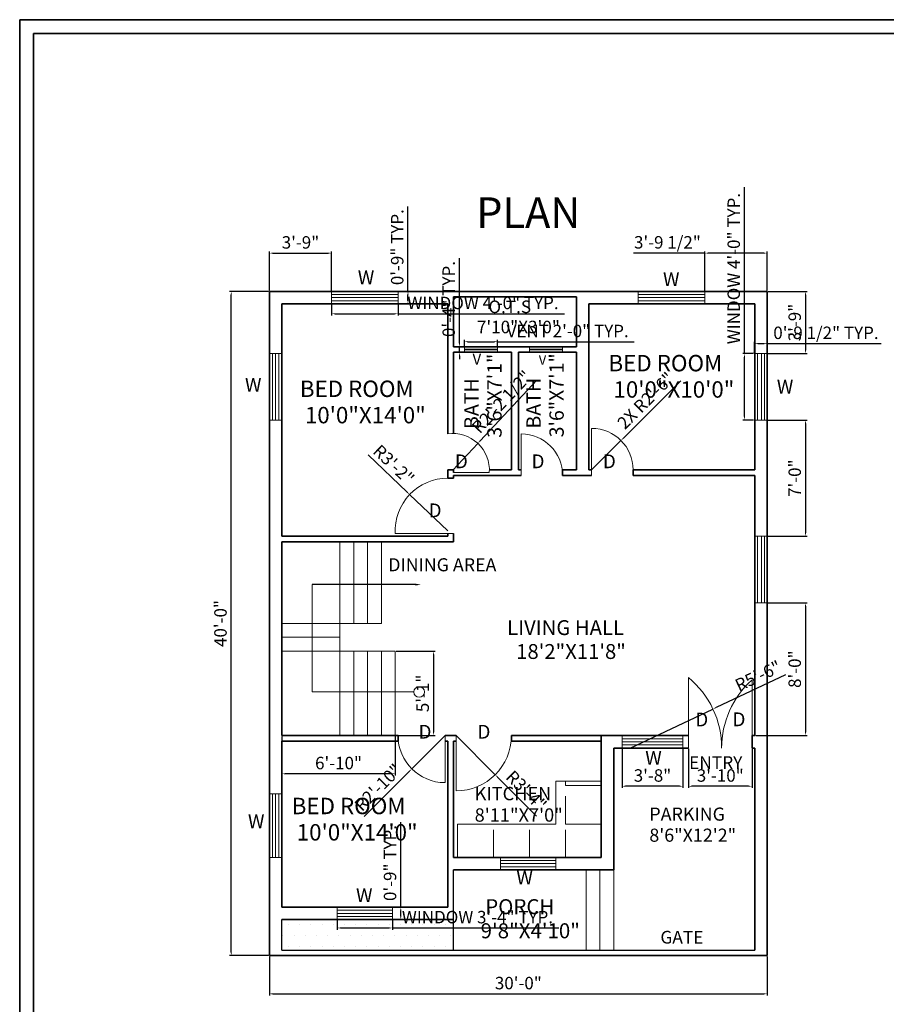
# Model space of a CAD drawing. Units: inches. Extents: x 2413 to 4117, y 1127 to 2321.
# Tile 3 of 5: x 2413 to 3039, y 1610 to 2321. Entities that reach past the tile are written whole.
import ezdxf
from ezdxf import colors
from ezdxf.entities.mleader import LeaderData, LeaderLine
from ezdxf.math import Vec2, Vec3

# ---------------------------------------------------------------- set-up
doc = ezdxf.new("R2010")
doc.units = ezdxf.units.IN
doc.linetypes.add('ACAD_ISO02W100', pattern=[15, 12, -3])
doc.linetypes.add('ACAD_ISO03W100', pattern=[30, 12, -18])
doc.layers.get('Defpoints').update_dxf_attribs({"linetype": 'ACAD_ISO03W100'})
for name, color, linetype, lineweight in [('A-ANNO-DIMS', 2, 'Continuous', 18), ('A-ANNO-SYMB', 2, 'Continuous', 18), ('A-ANNO-TEXT', 7, 'Continuous', 18), ('A-ANNO-TITL', 7, 'Continuous', 30), ('A-ANNO-TTLB', 7, 'Continuous', 35), ('A-AREA-IDEN', 7, 'Continuous', 18), ('A-DOOR', 3, 'Continuous', 20), ('A-FLOR', 7, 'Continuous', 30), ('A-FLOR-FIXT', 8, 'Continuous', 18), ('A-FLOR-OVHD', 8, 'ACAD_ISO02W100', 18), ('A-FLOR-PATT', 4, 'Continuous', 13), ('A-FLOR-STRS', 3, 'Continuous', 20), ('A-GLAZ', 4, 'Continuous', 18), ('A-WALL', 7, 'Continuous', 35)]:
    doc.layers.add(name, color=color, linetype=linetype, lineweight=lineweight)
doc.styles.get("Standard").update_dxf_attribs({"font": 'arial.ttf'})
doc.dimstyles.new('ISO-25', dxfattribs={"dimtxt": 9, "dimasz": 2.5, "dimexe": 1.25, "dimexo": 0.625, "dimgap": 2, "dimtad": 1, "dimdec": 1, "dimlunit": 4, "dimtxsty": 'Standard', "dimcen": 2.5, "dimazin": 0, "dimtfac": 1, "dimtdec": 1, "dimtmove": 0, "dimatfit": 3, "dimfxl": 1, "dimarcsym": 0})

# ---------------------------------------------------------------- blocks, each defined once
blk = doc.blocks.new('WIN-48-PLAN')
for p, q in [((0, 9), (0, 0)), ((48, 9), (48, 0)), ((0, 6.75), (48, 6.75)), ((0, 4.5), (48, 4.5)), ((0, 2.25), (48, 2.25))]:
    blk.add_line(p, q)
blk = doc.blocks.new('WIN-40-PLAN')
for p, q in [((0, 0), (0, 9)), ((40, 0), (40, 9)), ((0, 6.75), (40, 6.75)), ((0, 4.5), (40, 4.5)), ((0, 2.25), (40, 2.25))]:
    blk.add_line(p, q)
blk = doc.blocks.new('VENT-24-PLAN')
for p, q in [((0, 0), (0, 4)), ((0, 2.25), (24, 2.25)), ((0, 1.75), (24, 1.75)), ((24, 0), (24, 4))]:
    blk.add_line(p, q)
blk = doc.blocks.new('WIN-48-SIDE-PLAN')
for p, q in [((0, 48), (9.25, 48)), ((2.25, 48), (2.25, 0)), ((5, 48), (5, 0)), ((7.25, 48), (7.25, 0)), ((0, 0), (9.25, 0))]:
    blk.add_line(p, q)
blk = doc.blocks.new('*D16')
at = {"layer": 'A-ANNO-DIMS', "color": 0, "lineweight": -2, "transparency": 16777216}
for p, q in [((2638.17, 2115.41), (2638.17, 2107.58)), ((2686.17, 2115.41), (2686.17, 2107.58)), ((2640.67, 2108.83), (2683.67, 2108.83)), ((2686.17, 2108.83), (2806.56, 2108.83))]:
    blk.add_line(p, q, dxfattribs=at)
at = {"layer": 'A-ANNO-DIMS', "color": 0, "transparency": 16777216}
for points in [[(2640.67, 2109.25), (2640.67, 2108.42), (2638.17, 2108.83)], [(2683.67, 2109.25), (2683.67, 2108.42), (2686.17, 2108.83)]]:
    blk.add_solid(points, dxfattribs=at)
at = {"layer": 'Defpoints', "color": 0, "transparency": 16777216}
for p in [(2638.17, 2116.03), (2686.17, 2116.03), (2686.17, 2108.83)]:
    blk.add_point(p, dxfattribs=at)
at = {"layer": 'A-ANNO-DIMS', "color": 0, "transparency": 16777216, "insert": (2747.61, 2115.49), "char_height": 9, "attachment_point": 5}
blk.add_mtext('WINDOW 4\'-0" TYP.', dxfattribs=at)
blk = doc.blocks.new('*D17')
at = {"layer": 'A-ANNO-DIMS', "color": 0, "lineweight": -2, "transparency": 16777216}
for p, q in [((2693.37, 2125.03), (2693.37, 2186.39)), ((2686.79, 2125.03), (2694.62, 2125.03)), ((2693.37, 2118.53), (2693.37, 2122.53)), ((2686.79, 2116.03), (2694.62, 2116.03))]:
    blk.add_line(p, q, dxfattribs=at)
at = {"layer": 'A-ANNO-DIMS', "color": 0, "transparency": 16777216}
for points in [[(2692.95, 2122.53), (2693.79, 2122.53), (2693.37, 2125.03)], [(2692.95, 2118.53), (2693.79, 2118.53), (2693.37, 2116.03)]]:
    blk.add_solid(points, dxfattribs=at)
at = {"layer": 'Defpoints', "color": 0, "transparency": 16777216}
for p in [(2686.17, 2125.03), (2693.37, 2125.03), (2686.17, 2116.03)]:
    blk.add_point(p, dxfattribs=at)
at = {"layer": 'A-ANNO-DIMS', "color": 0, "transparency": 16777216, "insert": (2686.77, 2156.96), "char_height": 9, "attachment_point": 5, "rotation": 90}
blk.add_mtext('0\'-9" TYP.', dxfattribs=at)
blk = doc.blocks.new('*D18')
at = {"layer": 'A-ANNO-DIMS', "color": 0, "lineweight": -2, "transparency": 16777216}
for p, q in [((2642.17, 1670.41), (2642.17, 1663.78)), ((2644.67, 1665.03), (2679.67, 1665.03)), ((2682.17, 1670.41), (2682.17, 1663.78)), ((2682.17, 1665.03), (2802.56, 1665.03))]:
    blk.add_line(p, q, dxfattribs=at)
at = {"layer": 'A-ANNO-DIMS', "color": 0, "transparency": 16777216}
for points in [[(2644.67, 1665.45), (2644.67, 1664.62), (2642.17, 1665.03)], [(2679.67, 1665.45), (2679.67, 1664.62), (2682.17, 1665.03)]]:
    blk.add_solid(points, dxfattribs=at)
at = {"layer": 'Defpoints', "color": 0, "transparency": 16777216}
for p in [(2642.17, 1671.03), (2682.17, 1671.03), (2682.17, 1665.03)]:
    blk.add_point(p, dxfattribs=at)
at = {"layer": 'A-ANNO-DIMS', "color": 0, "transparency": 16777216, "insert": (2743.61, 1671.69), "char_height": 9, "attachment_point": 5}
blk.add_mtext('WINDOW 3\'-4" TYP.', dxfattribs=at)
blk = doc.blocks.new('*D19')
at = {"layer": 'A-ANNO-DIMS', "color": 0, "lineweight": -2, "transparency": 16777216}
for p, q in [((2688.17, 1680.03), (2688.17, 1741.39)), ((2682.79, 1680.03), (2689.42, 1680.03)), ((2688.17, 1673.53), (2688.17, 1677.53)), ((2682.79, 1671.03), (2689.42, 1671.03))]:
    blk.add_line(p, q, dxfattribs=at)
at = {"layer": 'A-ANNO-DIMS', "color": 0, "transparency": 16777216}
for points in [[(2687.75, 1677.53), (2688.59, 1677.53), (2688.17, 1680.03)], [(2687.75, 1673.53), (2688.59, 1673.53), (2688.17, 1671.03)]]:
    blk.add_solid(points, dxfattribs=at)
at = {"layer": 'Defpoints', "color": 0, "transparency": 16777216}
for p in [(2682.17, 1680.03), (2688.17, 1680.03), (2682.17, 1671.03)]:
    blk.add_point(p, dxfattribs=at)
at = {"layer": 'A-ANNO-DIMS', "color": 0, "transparency": 16777216, "insert": (2681.57, 1711.96), "char_height": 9, "attachment_point": 5, "rotation": 90}
blk.add_mtext('0\'-9" TYP.', dxfattribs=at)
blk = doc.blocks.new('*D20')
at = {"layer": 'A-ANNO-DIMS', "color": 0, "lineweight": -2, "transparency": 16777216}
for p, q in [((2734.17, 2085.66), (2734.17, 2089.88)), ((2736.67, 2088.63), (2755.67, 2088.63)), ((2758.17, 2085.66), (2758.17, 2089.88)), ((2758.17, 2088.63), (2857.02, 2088.63))]:
    blk.add_line(p, q, dxfattribs=at)
at = {"layer": 'A-ANNO-DIMS', "color": 0, "transparency": 16777216}
for points in [[(2736.67, 2089.05), (2736.67, 2088.22), (2734.17, 2088.63)], [(2755.67, 2089.05), (2755.67, 2088.22), (2758.17, 2088.63)]]:
    blk.add_solid(points, dxfattribs=at)
at = {"layer": 'Defpoints', "color": 0, "transparency": 16777216}
for p in [(2734.17, 2085.03), (2758.17, 2088.63), (2758.17, 2085.03)]:
    blk.add_point(p, dxfattribs=at)
at = {"layer": 'A-ANNO-DIMS', "color": 0, "transparency": 16777216, "insert": (2808.84, 2095.23), "char_height": 9, "attachment_point": 5}
blk.add_mtext('VENT 2\'-0" TYP.', dxfattribs=at)
blk = doc.blocks.new('*D21')
at = {"layer": 'A-ANNO-DIMS', "color": 0, "lineweight": -2, "transparency": 16777216}
for p, q in [((2730.57, 2087.53), (2730.57, 2148.89)), ((2733.54, 2085.03), (2729.32, 2085.03)), ((2730.57, 2081.03), (2730.57, 2085.03)), ((2733.54, 2081.03), (2729.32, 2081.03)), ((2730.57, 2078.53), (2730.57, 2076.03))]:
    blk.add_line(p, q, dxfattribs=at)
at = {"layer": 'A-ANNO-DIMS', "color": 0, "transparency": 16777216}
for points in [[(2730.15, 2087.53), (2730.99, 2087.53), (2730.57, 2085.03)], [(2730.15, 2078.53), (2730.99, 2078.53), (2730.57, 2081.03)]]:
    blk.add_solid(points, dxfattribs=at)
at = {"layer": 'Defpoints', "color": 0, "transparency": 16777216}
for p in [(2730.57, 2085.03), (2734.17, 2085.03), (2734.17, 2081.03)]:
    blk.add_point(p, dxfattribs=at)
at = {"layer": 'A-ANNO-DIMS', "color": 0, "transparency": 16777216, "insert": (2723.97, 2119.46), "char_height": 9, "attachment_point": 5, "rotation": 90}
blk.add_mtext('0\'-4" TYP.', dxfattribs=at)
blk = doc.blocks.new('*D22')
at = {"layer": 'A-ANNO-DIMS', "color": 0, "lineweight": -2, "transparency": 16777216}
for p, q in [((2936.72, 2080.03), (2936.72, 2200.42)), ((2943.29, 2080.03), (2935.47, 2080.03)), ((2936.72, 2034.53), (2936.72, 2077.53)), ((2943.29, 2032.03), (2935.47, 2032.03))]:
    blk.add_line(p, q, dxfattribs=at)
at = {"layer": 'A-ANNO-DIMS', "color": 0, "transparency": 16777216}
for points in [[(2936.3, 2077.53), (2937.14, 2077.53), (2936.72, 2080.03)], [(2936.3, 2034.53), (2937.14, 2034.53), (2936.72, 2032.03)]]:
    blk.add_solid(points, dxfattribs=at)
at = {"layer": 'Defpoints', "color": 0, "transparency": 16777216}
for p in [(2936.72, 2080.03), (2943.92, 2080.03), (2943.92, 2032.03)]:
    blk.add_point(p, dxfattribs=at)
at = {"layer": 'A-ANNO-DIMS', "color": 0, "transparency": 16777216, "insert": (2930.06, 2141.48), "char_height": 9, "attachment_point": 5, "rotation": 90}
blk.add_mtext('WINDOW 4\'-0" TYP.', dxfattribs=at)
blk = doc.blocks.new('*D23')
at = {"layer": 'A-ANNO-DIMS', "color": 0, "lineweight": -2, "transparency": 16777216}
for p, q in [((2943.92, 2080.66), (2943.92, 2088.48)), ((2946.42, 2087.23), (2950.67, 2087.23)), ((2953.17, 2080.66), (2953.17, 2088.48)), ((2953.17, 2087.23), (3035.5, 2087.23))]:
    blk.add_line(p, q, dxfattribs=at)
at = {"layer": 'A-ANNO-DIMS', "color": 0, "transparency": 16777216}
for points in [[(2946.42, 2087.65), (2946.42, 2086.82), (2943.92, 2087.23)], [(2950.67, 2087.65), (2950.67, 2086.82), (2953.17, 2087.23)]]:
    blk.add_solid(points, dxfattribs=at)
at = {"layer": 'Defpoints', "color": 0, "transparency": 16777216}
for p in [(2953.17, 2087.23), (2943.92, 2080.03), (2953.17, 2080.03)]:
    blk.add_point(p, dxfattribs=at)
at = {"layer": 'A-ANNO-DIMS', "color": 0, "transparency": 16777216, "insert": (2995.58, 2093.89), "char_height": 9, "attachment_point": 5}
blk.add_mtext('0\'-9 1/2" TYP.', dxfattribs=at)
blk = doc.blocks.new('*D32')
at = {"layer": 'A-ANNO-DIMS', "color": 0, "lineweight": -2, "transparency": 16777216}
for p, q in [((2593.17, 1644.41), (2593.17, 1616.18)), ((2953.17, 1644.41), (2953.17, 1616.18)), ((2595.67, 1617.43), (2950.67, 1617.43))]:
    blk.add_line(p, q, dxfattribs=at)
at = {"layer": 'A-ANNO-DIMS', "color": 0, "transparency": 16777216}
for points in [[(2595.67, 1617.85), (2595.67, 1617.02), (2593.17, 1617.43)], [(2950.67, 1617.85), (2950.67, 1617.02), (2953.17, 1617.43)]]:
    blk.add_solid(points, dxfattribs=at)
at = {"layer": 'Defpoints', "color": 0, "transparency": 16777216}
for p in [(2593.17, 1645.03), (2953.17, 1645.03), (2953.17, 1617.43)]:
    blk.add_point(p, dxfattribs=at)
at = {"layer": 'A-ANNO-DIMS', "color": 0, "transparency": 16777216, "insert": (2773.17, 1624.03), "char_height": 9, "attachment_point": 5}
blk.add_mtext('30\'-0"', dxfattribs=at)
blk = doc.blocks.new('*D33')
at = {"layer": 'A-ANNO-DIMS', "color": 0, "lineweight": -2, "transparency": 16777216}
for p, q in [((2592.54, 2125.03), (2564.32, 2125.03)), ((2565.57, 1647.53), (2565.57, 2122.53)), ((2592.54, 1645.03), (2564.32, 1645.03))]:
    blk.add_line(p, q, dxfattribs=at)
at = {"layer": 'A-ANNO-DIMS', "color": 0, "transparency": 16777216}
for points in [[(2565.15, 2122.53), (2565.99, 2122.53), (2565.57, 2125.03)], [(2565.15, 1647.53), (2565.99, 1647.53), (2565.57, 1645.03)]]:
    blk.add_solid(points, dxfattribs=at)
at = {"layer": 'Defpoints', "color": 0, "transparency": 16777216}
for p in [(2565.57, 2125.03), (2593.17, 2125.03), (2593.17, 1645.03)]:
    blk.add_point(p, dxfattribs=at)
at = {"layer": 'A-ANNO-DIMS', "color": 0, "transparency": 16777216, "insert": (2558.97, 1885.03), "char_height": 9, "attachment_point": 5, "rotation": 90}
blk.add_mtext('40\'-0"', dxfattribs=at)
blk = doc.blocks.new('*D34')
at = {"layer": 'A-ANNO-DIMS', "color": 0, "lineweight": -2, "transparency": 16777216}
for p, q in [((2593.17, 2125.66), (2593.17, 2153.88)), ((2595.67, 2152.63), (2635.67, 2152.63)), ((2638.17, 2125.66), (2638.17, 2153.88))]:
    blk.add_line(p, q, dxfattribs=at)
at = {"layer": 'A-ANNO-DIMS', "color": 0, "transparency": 16777216}
for points in [[(2595.67, 2153.05), (2595.67, 2152.22), (2593.17, 2152.63)], [(2635.67, 2153.05), (2635.67, 2152.22), (2638.17, 2152.63)]]:
    blk.add_solid(points, dxfattribs=at)
at = {"layer": 'Defpoints', "color": 0, "transparency": 16777216}
for p in [(2638.17, 2152.63), (2593.17, 2125.03), (2638.17, 2125.03)]:
    blk.add_point(p, dxfattribs=at)
at = {"layer": 'A-ANNO-DIMS', "color": 0, "transparency": 16777216, "insert": (2615.67, 2159.23), "char_height": 9, "attachment_point": 5}
blk.add_mtext('3\'-9"', dxfattribs=at)
blk = doc.blocks.new('*D35')
at = {"layer": 'A-ANNO-DIMS', "color": 0, "lineweight": -2, "transparency": 16777216}
for p, q in [((2907.92, 2152.63), (2856.53, 2152.63)), ((2907.92, 2125.66), (2907.92, 2153.88)), ((2950.67, 2152.63), (2910.42, 2152.63)), ((2953.17, 2125.66), (2953.17, 2153.88))]:
    blk.add_line(p, q, dxfattribs=at)
at = {"layer": 'A-ANNO-DIMS', "color": 0, "transparency": 16777216}
for points in [[(2910.42, 2153.05), (2910.42, 2152.22), (2907.92, 2152.63)], [(2950.67, 2153.05), (2950.67, 2152.22), (2953.17, 2152.63)]]:
    blk.add_solid(points, dxfattribs=at)
at = {"layer": 'Defpoints', "color": 0, "transparency": 16777216}
for p in [(2907.92, 2152.63), (2907.92, 2125.03), (2953.17, 2125.03)]:
    blk.add_point(p, dxfattribs=at)
at = {"layer": 'A-ANNO-DIMS', "color": 0, "transparency": 16777216, "insert": (2880.97, 2159.29), "char_height": 9, "attachment_point": 5}
blk.add_mtext('3\'-9 1/2"', dxfattribs=at)
blk = doc.blocks.new('*D36')
at = {"layer": 'A-ANNO-DIMS', "color": 0, "lineweight": -2, "transparency": 16777216}
for p, q in [((2953.79, 2125.03), (2982.02, 2125.03)), ((2980.77, 2122.53), (2980.77, 2082.53)), ((2953.79, 2080.03), (2982.02, 2080.03))]:
    blk.add_line(p, q, dxfattribs=at)
at = {"layer": 'A-ANNO-DIMS', "color": 0, "transparency": 16777216}
for points in [[(2980.35, 2122.53), (2981.19, 2122.53), (2980.77, 2125.03)], [(2980.35, 2082.53), (2981.19, 2082.53), (2980.77, 2080.03)]]:
    blk.add_solid(points, dxfattribs=at)
at = {"layer": 'Defpoints', "color": 0, "transparency": 16777216}
for p in [(2953.17, 2125.03), (2953.17, 2080.03), (2980.77, 2080.03)]:
    blk.add_point(p, dxfattribs=at)
at = {"layer": 'A-ANNO-DIMS', "color": 0, "transparency": 16777216, "insert": (2974.17, 2102.53), "char_height": 9, "attachment_point": 5, "rotation": 90}
blk.add_mtext('3\'-9"', dxfattribs=at)
blk = doc.blocks.new('*D37')
at = {"layer": 'A-ANNO-DIMS', "color": 0, "lineweight": -2, "transparency": 16777216}
for p, q in [((2953.79, 2032.03), (2982.02, 2032.03)), ((2980.77, 2029.53), (2980.77, 1950.53)), ((2953.79, 1948.03), (2982.02, 1948.03))]:
    blk.add_line(p, q, dxfattribs=at)
at = {"layer": 'A-ANNO-DIMS', "color": 0, "transparency": 16777216}
for points in [[(2980.35, 2029.53), (2981.19, 2029.53), (2980.77, 2032.03)], [(2980.35, 1950.53), (2981.19, 1950.53), (2980.77, 1948.03)]]:
    blk.add_solid(points, dxfattribs=at)
at = {"layer": 'Defpoints', "color": 0, "transparency": 16777216}
for p in [(2953.17, 2032.03), (2953.17, 1948.03), (2980.77, 1948.03)]:
    blk.add_point(p, dxfattribs=at)
at = {"layer": 'A-ANNO-DIMS', "color": 0, "transparency": 16777216, "insert": (2974.17, 1990.03), "char_height": 9, "attachment_point": 5, "rotation": 90}
blk.add_mtext('7\'-0"', dxfattribs=at)
blk = doc.blocks.new('*D38')
at = {"layer": 'A-ANNO-DIMS', "color": 0, "lineweight": -2, "transparency": 16777216}
for p, q in [((2953.79, 1900.03), (2982.02, 1900.03)), ((2980.77, 1897.53), (2980.77, 1806.53)), ((2944.79, 1804.03), (2982.02, 1804.03))]:
    blk.add_line(p, q, dxfattribs=at)
at = {"layer": 'A-ANNO-DIMS', "color": 0, "transparency": 16777216}
for points in [[(2980.35, 1897.53), (2981.19, 1897.53), (2980.77, 1900.03)], [(2980.35, 1806.53), (2981.19, 1806.53), (2980.77, 1804.03)]]:
    blk.add_solid(points, dxfattribs=at)
at = {"layer": 'Defpoints', "color": 0, "transparency": 16777216}
for p in [(2953.17, 1900.03), (2944.17, 1804.03), (2980.77, 1804.03)]:
    blk.add_point(p, dxfattribs=at)
at = {"layer": 'A-ANNO-DIMS', "color": 0, "transparency": 16777216, "insert": (2974.17, 1852.03), "char_height": 9, "attachment_point": 5, "rotation": 90}
blk.add_mtext('8\'-0"', dxfattribs=at)
blk = doc.blocks.new('*D39')
at = {"layer": 'A-ANNO-DIMS', "color": 0, "lineweight": -2, "transparency": 16777216}
for p, q in [((2602.17, 1803.41), (2602.17, 1775.18)), ((2684.17, 1803.41), (2684.17, 1775.18)), ((2681.67, 1776.43), (2604.67, 1776.43))]:
    blk.add_line(p, q, dxfattribs=at)
at = {"layer": 'A-ANNO-DIMS', "color": 0, "transparency": 16777216}
for points in [[(2604.67, 1776.85), (2604.67, 1776.02), (2602.17, 1776.43)], [(2681.67, 1776.85), (2681.67, 1776.02), (2684.17, 1776.43)]]:
    blk.add_solid(points, dxfattribs=at)
at = {"layer": 'Defpoints', "color": 0, "transparency": 16777216}
for p in [(2602.17, 1804.03), (2684.17, 1804.03), (2602.17, 1776.43)]:
    blk.add_point(p, dxfattribs=at)
at = {"layer": 'A-ANNO-DIMS', "color": 0, "transparency": 16777216, "insert": (2643.17, 1783.03), "char_height": 9, "attachment_point": 5}
blk.add_mtext('6\'-10"', dxfattribs=at)
blk = doc.blocks.new('*D40')
at = {"layer": 'A-ANNO-DIMS', "color": 0, "lineweight": -2, "transparency": 16777216}
for p, q in [((2684.79, 1865.03), (2713.02, 1865.03)), ((2711.77, 1862.53), (2711.77, 1806.53)), ((2684.79, 1804.03), (2713.02, 1804.03))]:
    blk.add_line(p, q, dxfattribs=at)
at = {"layer": 'A-ANNO-DIMS', "color": 0, "transparency": 16777216}
for points in [[(2711.35, 1862.53), (2712.19, 1862.53), (2711.77, 1865.03)], [(2711.35, 1806.53), (2712.19, 1806.53), (2711.77, 1804.03)]]:
    blk.add_solid(points, dxfattribs=at)
at = {"layer": 'Defpoints', "color": 0, "transparency": 16777216}
for p in [(2684.17, 1865.03), (2684.17, 1804.03), (2711.77, 1804.03)]:
    blk.add_point(p, dxfattribs=at)
at = {"layer": 'A-ANNO-DIMS', "color": 0, "transparency": 16777216, "insert": (2705.17, 1834.53), "char_height": 9, "attachment_point": 5, "rotation": 90}
blk.add_mtext('5\'-1"', dxfattribs=at)
blk = doc.blocks.new('*D41')
at = {"layer": 'A-ANNO-DIMS', "color": 0, "lineweight": -2, "transparency": 16777216}
for p, q in [((2848.17, 1794.41), (2848.17, 1766.18)), ((2892.17, 1794.41), (2892.17, 1766.18)), ((2889.67, 1767.43), (2850.67, 1767.43))]:
    blk.add_line(p, q, dxfattribs=at)
at = {"layer": 'A-ANNO-DIMS', "color": 0, "transparency": 16777216}
for points in [[(2850.67, 1767.85), (2850.67, 1767.02), (2848.17, 1767.43)], [(2889.67, 1767.85), (2889.67, 1767.02), (2892.17, 1767.43)]]:
    blk.add_solid(points, dxfattribs=at)
at = {"layer": 'Defpoints', "color": 0, "transparency": 16777216}
for p in [(2848.17, 1795.03), (2892.17, 1795.03), (2848.17, 1767.43)]:
    blk.add_point(p, dxfattribs=at)
at = {"layer": 'A-ANNO-DIMS', "color": 0, "transparency": 16777216, "insert": (2870.17, 1774.03), "char_height": 9, "attachment_point": 5}
blk.add_mtext('3\'-8"', dxfattribs=at)
blk = doc.blocks.new('*D42')
at = {"layer": 'A-ANNO-DIMS', "color": 0, "lineweight": -2, "transparency": 16777216}
for p, q in [((2896.17, 1794.41), (2896.17, 1766.18)), ((2942.17, 1794.41), (2942.17, 1766.18)), ((2939.67, 1767.43), (2898.67, 1767.43))]:
    blk.add_line(p, q, dxfattribs=at)
at = {"layer": 'A-ANNO-DIMS', "color": 0, "transparency": 16777216}
for points in [[(2898.67, 1767.85), (2898.67, 1767.02), (2896.17, 1767.43)], [(2939.67, 1767.85), (2939.67, 1767.02), (2942.17, 1767.43)]]:
    blk.add_solid(points, dxfattribs=at)
at = {"layer": 'Defpoints', "color": 0, "transparency": 16777216}
for p in [(2896.17, 1795.03), (2942.17, 1795.03), (2896.17, 1767.43)]:
    blk.add_point(p, dxfattribs=at)
at = {"layer": 'A-ANNO-DIMS', "color": 0, "transparency": 16777216, "insert": (2919.17, 1774.03), "char_height": 9, "attachment_point": 5}
blk.add_mtext('3\'-10"', dxfattribs=at)
blk = doc.blocks.new('*D88')
at = {"layer": 'A-ANNO-DIMS', "color": 0, "lineweight": -2, "transparency": 16777216}
for p, q in [((2966.33, 1847.9), (2916.13, 1824.28)), ((2853.98, 1795.03), (2913.87, 1823.21))]:
    blk.add_line(p, q, dxfattribs=at)
at = {"layer": 'A-ANNO-DIMS', "color": 0, "transparency": 16777216}
blk.add_solid([(2915.95, 1824.66), (2916.31, 1823.9), (2913.87, 1823.21)], dxfattribs=at)
at = {"layer": 'Defpoints', "color": 0, "transparency": 16777216}
for p in [(2913.87, 1823.21), (2853.98, 1795.03)]:
    blk.add_point(p, dxfattribs=at)
at = {"layer": 'A-ANNO-DIMS', "color": 0, "transparency": 16777216, "insert": (2946.99, 1846.09), "char_height": 9, "attachment_point": 5, "rotation": 25.20091}
blk.add_mtext('R5\'-6"', dxfattribs=at)
blk = doc.blocks.new('*D89')
at = {"layer": 'A-ANNO-DIMS', "color": 0, "lineweight": -2, "transparency": 16777216}
for p, q in [((2728.17, 1804.03), (2756.45, 1775.75)), ((2786.34, 1745.86), (2758.22, 1773.98))]:
    blk.add_line(p, q, dxfattribs=at)
at = {"layer": 'A-ANNO-DIMS', "color": 0, "transparency": 16777216}
blk.add_solid([(2758.52, 1774.27), (2757.93, 1773.69), (2756.45, 1775.75)], dxfattribs=at)
at = {"layer": 'Defpoints', "color": 0, "transparency": 16777216}
for p in [(2728.17, 1804.03), (2756.45, 1775.75)]:
    blk.add_point(p, dxfattribs=at)
at = {"layer": 'A-ANNO-DIMS', "color": 0, "transparency": 16777216, "insert": (2778.09, 1763.44), "char_height": 9, "attachment_point": 5, "rotation": 315.00027}
blk.add_mtext('R3\'-4"', dxfattribs=at)
blk = doc.blocks.new('*D90')
at = {"layer": 'A-ANNO-DIMS', "color": 0, "lineweight": -2, "transparency": 16777216}
for p, q in [((2664.47, 2006.8), (2692.77, 1979.91)), ((2722.17, 1951.98), (2694.58, 1978.19))]:
    blk.add_line(p, q, dxfattribs=at)
at = {"layer": 'A-ANNO-DIMS', "color": 0, "transparency": 16777216}
blk.add_solid([(2693.06, 1980.21), (2692.48, 1979.61), (2694.58, 1978.19)], dxfattribs=at)
at = {"layer": 'Defpoints', "color": 0, "transparency": 16777216}
for p in [(2694.58, 1978.19), (2722.17, 1951.98)]:
    blk.add_point(p, dxfattribs=at)
at = {"layer": 'A-ANNO-DIMS', "color": 0, "transparency": 16777216, "insert": (2682.26, 1999), "char_height": 9, "attachment_point": 5, "rotation": 316.46818}
blk.add_mtext('R3\'-2"', dxfattribs=at)
blk = doc.blocks.new('*D91')
at = {"layer": 'A-ANNO-DIMS', "color": 0, "lineweight": -2, "transparency": 16777216}
for p, q in [((2720.17, 1804.03), (2696.13, 1779.99)), ((2661.81, 1745.67), (2694.36, 1778.22))]:
    blk.add_line(p, q, dxfattribs=at)
at = {"layer": 'A-ANNO-DIMS', "color": 0, "transparency": 16777216}
blk.add_solid([(2694.06, 1778.52), (2694.65, 1777.93), (2696.13, 1779.99)], dxfattribs=at)
at = {"layer": 'Defpoints', "color": 0, "transparency": 16777216}
for p in [(2720.17, 1804.03), (2696.13, 1779.99)]:
    blk.add_point(p, dxfattribs=at)
at = {"layer": 'A-ANNO-DIMS', "color": 0, "transparency": 16777216, "insert": (2672.54, 1765.73), "char_height": 9, "attachment_point": 5, "rotation": 44.99999}
blk.add_mtext('R2\'-10"', dxfattribs=at)
blk = doc.blocks.new('*D92')
at = {"layer": 'A-ANNO-DIMS', "color": 0, "lineweight": -2, "transparency": 16777216}
for p, q in [((2890.54, 2060.4), (2849.15, 2019.01)), ((2826.17, 1996.03), (2847.38, 2017.25))]:
    blk.add_line(p, q, dxfattribs=at)
at = {"layer": 'A-ANNO-DIMS', "color": 0, "transparency": 16777216}
blk.add_solid([(2848.86, 2019.31), (2849.44, 2018.72), (2847.38, 2017.25)], dxfattribs=at)
at = {"layer": 'Defpoints', "color": 0, "transparency": 16777216}
for p in [(2847.38, 2017.25), (2826.17, 1996.03)]:
    blk.add_point(p, dxfattribs=at)
at = {"layer": 'A-ANNO-DIMS', "color": 0, "transparency": 16777216, "insert": (2866.06, 2045.25), "char_height": 9, "attachment_point": 5, "rotation": 45.00001}
blk.add_mtext('2X R2\'-6"', dxfattribs=at)
blk = doc.blocks.new('*D93')
at = {"layer": 'A-ANNO-DIMS', "color": 0, "lineweight": -2, "transparency": 16777216}
for p, q in [((2786.51, 2060.9), (2745.57, 2017.03)), ((2725.87, 1995.93), (2743.86, 2015.2))]:
    blk.add_line(p, q, dxfattribs=at)
at = {"layer": 'A-ANNO-DIMS', "color": 0, "transparency": 16777216}
blk.add_solid([(2745.26, 2017.31), (2745.87, 2016.75), (2743.86, 2015.2)], dxfattribs=at)
at = {"layer": 'Defpoints', "color": 0, "transparency": 16777216}
for p in [(2743.86, 2015.2), (2725.87, 1995.93)]:
    blk.add_point(p, dxfattribs=at)
at = {"layer": 'A-ANNO-DIMS', "color": 0, "transparency": 16777216, "insert": (2762.03, 2044.42), "char_height": 9, "attachment_point": 5, "rotation": 46.97493}
blk.add_mtext('R2\'-2 1/2"', dxfattribs=at)

msp = doc.modelspace()

# ---------------------------------------------------------------- hatches: boundary and pattern name
at = {"layer": 'A-FLOR-PATT'}
h = msp.add_hatch(dxfattribs=at)
h.set_pattern_fill('DOTS', color=256, scale=5.1)
h.paths.add_polyline_path([(2726.17, 1671.03), (2602.17, 1671.03), (2602.17, 1649.03), (2726.17, 1649.03)])

# ---------------------------------------------------------------- linework, layer by layer
at = {"layer": 'A-ANNO-SYMB'}
for q in [(2624.17, 1913.11), (2697.64, 1835.53)]:
    msp.add_line((2624.17, 1835.53), q, dxfattribs=at)
msp.add_circle((2701.48, 1835.53), 3.84, dxfattribs=at)
at = {"layer": 'A-ANNO-TTLB'}
for points in [[(2412.62, 2321.32), (4117.04, 2321.32), (4117.04, 1126.9), (2412.62, 1126.9)], [(2422.62, 2311.32), (4107.04, 2311.32), (4107.04, 1136.9), (2422.62, 1136.9)]]:
    msp.add_lwpolyline(points, close=True, dxfattribs=at)
at = {"layer": 'A-DOOR'}
for p, q in [((2775.17, 1992.03), (2775.17, 2022.03)), ((2826.17, 2026.03), (2826.17, 1992.03)), ((2726.17, 1994.03), (2752.17, 1994.03)), ((2684.17, 1950.03), (2726.17, 1950.03)), ((2896.17, 1846.03), (2896.17, 1795.03)), ((2942.17, 1844.08), (2942.17, 1804.03)), ((2720.17, 1770.03), (2720.17, 1804.03)), ((2728.17, 1764.03), (2728.17, 1804.03))]:
    msp.add_line(p, q, dxfattribs=at)
for centre, radius, start, end in [((2725.87, 1995.93), 26.37, 355.8767, 98.07316), ((2775.17, 1992.03), 30, 0, 90), ((2826.17, 1996.03), 30, 0, 90), ((2722.17, 1951.98), 38.05, 90, 182.9376), ((2853.98, 1795.03), 66.19, 0, 50.40225), ((2986.36, 1795.03), 66.19, 132.17429, 180), ((2720.17, 1804.03), 34, 180, 270), ((2728.17, 1804.03), 40, 270, 0)]:
    msp.add_arc(centre, radius, start, end, dxfattribs=at)
at = {"layer": 'A-FLOR'}
for p, q in [((2726.17, 1649.03), (2726.17, 1707.03)), ((2602.17, 1649.03), (2602.17, 1671.03)), ((2602.17, 1649.03), (2944.17, 1649.03))]:
    msp.add_line(p, q, dxfattribs=at)
at = {"layer": 'A-FLOR-FIXT'}
for p, q in [((2800.17, 1740.03), (2800.17, 1771.03)), ((2800.17, 1771.03), (2833.17, 1771.03)), ((2800.17, 1749.03), (2800.17, 1771.03)), ((2807.17, 1768.03), (2807.17, 1771.03)), ((2807.17, 1768.03), (2833.17, 1768.03)), ((2807.17, 1740.03), (2807.17, 1760.2)), ((2729.17, 1716.03), (2729.17, 1740.03)), ((2729.17, 1740.03), (2800.17, 1740.03)), ((2755.17, 1716.03), (2755.17, 1736.03)), ((2781.17, 1716.03), (2781.17, 1736.03)), ((2807.17, 1740.03), (2833.17, 1740.03)), ((2807.17, 1740.03), (2833.17, 1740.03)), ((2807.17, 1716.03), (2807.17, 1736.03))]:
    msp.add_line(p, q, dxfattribs=at)
at = {"layer": 'A-FLOR-OVHD'}
msp.add_line((2842.17, 1707.03), (2842.17, 1649.03), dxfattribs=at)
at = {"layer": 'A-FLOR-STRS'}
for p, q in [((2644.17, 1804.03), (2644.17, 1944.03)), ((2654.17, 1885.03), (2654.17, 1944.03)), ((2664.17, 1885.03), (2664.17, 1944.03)), ((2674.17, 1885.03), (2674.17, 1944.03)), ((2602.17, 1885.03), (2674.17, 1885.03)), ((2602.17, 1875.03), (2644.17, 1875.03)), ((2602.17, 1865.03), (2684.17, 1865.03)), ((2654.17, 1804.03), (2654.17, 1865.03)), ((2664.17, 1804.03), (2664.17, 1865.03)), ((2674.17, 1804.03), (2674.17, 1865.03)), ((2684.17, 1804.03), (2684.17, 1865.03)), ((2822.17, 1707.03), (2822.17, 1649.03)), ((2832.17, 1707.03), (2832.17, 1649.03)), ((2842.17, 1707.03), (2842.17, 1649.03))]:
    msp.add_line(p, q, dxfattribs=at)
at = {"layer": 'A-GLAZ'}
for p, q in [((2944.17, 1948.03), (2953.17, 1948.03)), ((2848.17, 1804.03), (2848.17, 1795.03)), ((2848.17, 1801.78), (2892.17, 1801.78)), ((2892.17, 1804.03), (2892.17, 1795.03)), ((2848.17, 1799.53), (2892.17, 1799.53)), ((2848.17, 1797.28), (2892.17, 1797.28)), ((2593.17, 1762.03), (2602.17, 1762.03)), ((2595.42, 1716.03), (2595.42, 1762.03)), ((2597.67, 1716.03), (2597.67, 1762.03)), ((2599.92, 1716.03), (2599.92, 1762.03)), ((2593.17, 1716.03), (2602.17, 1716.03))]:
    msp.add_line(p, q, dxfattribs=at)
at = {"layer": 'A-WALL'}
for p, q in [((2593.17, 2125.03), (2953.17, 2125.03)), ((2593.17, 1645.03), (2593.17, 2125.03)), ((2726.17, 2121.03), (2726.17, 2085.03)), ((2726.17, 2121.03), (2815.17, 2121.03)), ((2726.17, 2085.03), (2726.17, 2121.03)), ((2726.17, 2085.03), (2726.17, 2121.03)), ((2815.17, 2085.03), (2815.17, 2121.03)), ((2953.17, 2125.03), (2953.17, 1645.03)), ((2602.17, 2116.03), (2722.17, 2116.03)), ((2602.17, 1948.03), (2602.17, 2116.03)), ((2722.17, 2027.03), (2722.17, 2116.03)), ((2722.17, 2116.03), (2722.17, 2022.03)), ((2722.17, 2022.03), (2722.17, 2116.03)), ((2824.17, 2116.03), (2824.17, 1996.03)), ((2824.17, 2116.03), (2944.17, 2116.03)), ((2944.17, 2116.03), (2944.17, 1996.03)), ((2726.17, 2085.03), (2815.17, 2085.03)), ((2726.17, 2081.03), (2768.17, 2081.03)), ((2726.17, 2022.3), (2726.17, 2081.03)), ((2726.17, 2022.3), (2726.17, 2081.03)), ((2726.17, 2081.03), (2726.17, 2022.3)), ((2768.17, 1996.03), (2768.17, 2081.03)), ((2773.17, 1996.03), (2773.17, 2081.03)), ((2773.17, 2081.03), (2815.17, 2081.03)), ((2815.17, 1996.03), (2815.17, 2081.03)), ((2722.17, 1996.03), (2726.17, 1996.03)), ((2722.17, 1990.03), (2722.17, 1996.03)), ((2722.17, 1994.03), (2722.17, 1990.03)), ((2726.17, 1994.03), (2726.17, 1996.03)), ((2752.17, 1996.03), (2768.17, 1996.03)), ((2773.17, 1996.03), (2775.17, 1996.03)), ((2805.17, 1992.03), (2805.17, 1996.03)), ((2805.17, 1996.03), (2815.17, 1996.03)), ((2824.17, 1996.03), (2826.17, 1996.03)), ((2856.17, 1996.03), (2856.17, 1992.03)), ((2856.17, 1996.03), (2944.17, 1996.03)), ((2722.17, 1990.03), (2726.17, 1990.03)), ((2726.17, 1992.03), (2775.17, 1992.03)), ((2726.17, 1992.03), (2726.17, 1990.03)), ((2726.17, 1990.03), (2726.17, 1992.03)), ((2726.17, 1990.03), (2726.17, 1992.03)), ((2805.17, 1992.03), (2826.17, 1992.03)), ((2856.17, 1992.03), (2944.17, 1992.03)), ((2944.17, 1992.03), (2944.17, 1804.03)), ((2722.17, 1948.03), (2722.17, 1950.03)), ((2726.17, 1948.03), (2726.17, 1950.03)), ((2726.17, 1944.03), (2726.17, 1950.03)), ((2726.17, 1950.03), (2726.17, 1944.03)), ((2602.17, 1948.03), (2722.17, 1948.03)), ((2602.17, 1944.03), (2726.17, 1944.03)), ((2602.17, 1804.03), (2602.17, 1944.03)), ((2602.17, 1804.03), (2686.17, 1804.03)), ((2602.17, 1800.03), (2686.17, 1800.03)), ((2602.17, 1680.03), (2602.17, 1800.03)), ((2686.17, 1800.03), (2686.17, 1804.03)), ((2720.17, 1804.03), (2728.17, 1804.03)), ((2720.17, 1800.03), (2722.17, 1800.03)), ((2722.17, 1680.03), (2722.17, 1800.03)), ((2726.17, 1800.03), (2728.17, 1800.03)), ((2726.17, 1716.03), (2726.17, 1800.03)), ((2768.17, 1804.03), (2896.17, 1804.03)), ((2768.17, 1800.03), (2768.17, 1804.03)), ((2768.17, 1800.03), (2833.17, 1800.03)), ((2833.17, 1716.03), (2833.17, 1804.03)), ((2833.17, 1804.03), (2833.17, 1800.03)), ((2942.17, 1804.03), (2942.17, 1795.03)), ((2942.17, 1804.03), (2944.17, 1804.03)), ((2842.17, 1707.03), (2842.17, 1795.03)), ((2842.17, 1795.03), (2896.17, 1795.03)), ((2942.17, 1795.03), (2944.17, 1795.03)), ((2944.17, 1795.03), (2944.17, 1649.03)), ((2726.17, 1716.03), (2833.17, 1716.03)), ((2726.17, 1716.03), (2833.17, 1716.03)), ((2726.17, 1707.03), (2842.17, 1707.03)), ((2602.17, 1680.03), (2722.17, 1680.03)), ((2602.17, 1671.03), (2726.17, 1671.03)), ((2593.17, 1645.03), (2953.17, 1645.03))]:
    msp.add_line(p, q, dxfattribs=at)

# ---------------------------------------------------------------- block references
at = {"layer": 'A-GLAZ'}
for name, p in [('WIN-48-PLAN', (2638.17, 2116.03)), ('WIN-48-PLAN', (2859.92, 2116.03)), ('VENT-24-PLAN', (2734.17, 2081.03)), ('VENT-24-PLAN', (2781.17, 2081.03)), ('WIN-48-SIDE-PLAN', (2943.92, 2032.03)), ('WIN-48-SIDE-PLAN', (2943.92, 1900.03)), ('WIN-40-PLAN', (2760.17, 1707.03)), ('WIN-40-PLAN', (2642.17, 1671.03))]:
    msp.add_blockref(name, p, dxfattribs=at)
at = {"layer": 'A-GLAZ', "rotation": 90.00000000000254}
msp.add_blockref('WIN-48-PLAN', (2602.17, 2032.03), dxfattribs=at)

# ---------------------------------------------------------------- texts
at = {"layer": 'A-ANNO-TEXT'}
for s, height, p in [('W', 9.96, (2657.09, 2130.16)), ('W', 9.96, (2877.76, 2128.86)), ('V', 7.82, (2740.1, 2072.07)), ('V', 6.9, (2787.92, 2071.99)), ('W', 9.96, (2575.52, 2052.54)), ('W', 9.96, (2960.07, 2051.2)), ('D', 9.96, (2727.3, 1997.22)), ('D', 9.96, (2782.73, 1997.22)), ('D', 9.96, (2834.31, 1997.22)), ('D', 9.96, (2708.32, 1961.78)), ('D', 9.96, (2901.13, 1810.65)), ('D', 9.96, (2928.03, 1810.8)), ('D', 9.96, (2701.01, 1801.83)), ('D', 9.96, (2743.65, 1801.83)), ('W', 9.96, (2864.93, 1782.93)), ('ENTRY', 9.176, (2896.64, 1779.95)), ('W', 9.96, (2577.68, 1737.11)), ('W', 9.96, (2771.76, 1696.45)), ('W', 9.96, (2655.8, 1683.72)), ('GATE', 9.176, (2875.89, 1653.74))]:
    msp.add_text(s, height=height, dxfattribs=at).set_placement(p)
at = {"layer": 'A-ANNO-TITL'}
msp.add_text('PLAN', height=22.025, dxfattribs=at).set_placement((2742.68, 2170.92))
at = {"layer": 'A-AREA-IDEN'}
for s, height, p in [('   O.T.S', 9.073, (2743.2, 2109.31)), ('7\'10"X3\'0"', 9.073, (2743.2, 2094.73)), ('BED ROOM', 11.849, (2838.33, 2067.23)), ('BED ROOM', 11.849, (2615.21, 2048.69)), (' 10\'0"X10\'0"', 11.8492, (2838.33, 2048.2)), (' 10\'0"X14\'0"', 11.8492, (2615.21, 2029.66)), ('DINING AREA', 9.4376, (2679.1, 1922.74)), ('LIVING HALL', 10.7494, (2765.05, 1876.67)), ('  18\'2"X11\'8"', 10.7494, (2765.05, 1859.41)), ('KITCHEN', 9.629, (2741.58, 1757.3)), ('BED ROOM', 11.849, (2609.32, 1747.25)), ('8\'11"X7\'0"', 9.629, (2741.58, 1741.83)), ('PARKING', 9.479, (2867.9, 1742.55)), (' 10\'0"X14\'0"', 11.8492, (2609.32, 1728.21)), ('8\'6"X12\'2"', 9.479, (2867.9, 1727.32)), (' PORCH', 10.846, (2745.92, 1674.98)), ('9\'8"X4\'10"', 10.846, (2745.92, 1657.56))]:
    msp.add_text(s, height=height, dxfattribs=at).set_placement(p)
for s, p in [('3\'6"X7\'1"', (2761.08, 2019.23)), ('3\'6"X7\'1"', (2806, 2019.53)), ('  BATH', (2744.43, 2019.23)), ('  BATH', (2789.35, 2019.53))]:
    msp.add_text(s, height=10.362, rotation=90, dxfattribs=at).set_placement(p)

# ---------------------------------------------------------------- dimensions: what is measured, and where the dimension line sits
at = {"layer": 'A-ANNO-DIMS'}
for base, p1, p2, text, picture, middle in [((2936.72, 2080.03), (2943.92, 2032.03), (2943.92, 2080.03), 'WINDOW <> TYP.', '*D22', (2930.06, 2141.48)), ((2693.37, 2125.03), (2686.17, 2116.03), (2686.17, 2125.03), '<> TYP.', '*D17', (2686.77, 2156.96)), ((2730.57, 2085.03), (2734.17, 2081.03), (2734.17, 2085.03), '<> TYP.', '*D21', (2723.97, 2119.46)), ((2688.17, 1680.03), (2682.17, 1671.03), (2682.17, 1680.03), '<> TYP.', '*D19', (2681.57, 1711.96))]:
    dim = msp.add_linear_dim(base=base, p1=p1, p2=p2, angle=90, text=text, dimstyle='ISO-25', override={"dimdec": 1, "dimlfac": 1, "dimrnd": 0, "dimzin": 1, "dimdsep": 46, "dimlunit": 4, "dimfrac": 2}, dxfattribs=at)
    dim.commit()
    dim.dimension.update_dxf_attribs({"geometry": picture, "text_midpoint": middle})
for base, p1, p2, picture, middle in [((2907.918869, 2152.63186), (2953.168869, 2125.03186), (2907.918869, 2125.03186), '*D35', (2880.97412139, 2159.28840843)), ((2638.17, 2152.63), (2593.17, 2125.03), (2638.17, 2125.03), '*D34', (2615.67, 2159.23)), ((2953.17, 1617.43), (2593.17, 1645.03), (2953.17, 1645.03), '*D32', (2773.17, 1624.03))]:
    dim = msp.add_linear_dim(base=base, p1=p1, p2=p2, dimstyle='ISO-25', override={"dimdec": 1, "dimlfac": 1, "dimrnd": 0, "dimzin": 1, "dimdsep": 46, "dimlunit": 4, "dimfrac": 2}, dxfattribs=at)
    dim.commit()
    dim.dimension.update_dxf_attribs({"geometry": picture, "text_midpoint": middle})
for base, p1, p2, text, picture, middle in [((2686.17, 2108.83), (2638.17, 2116.03), (2686.17, 2116.03), 'WINDOW <> TYP.', '*D16', (2747.61, 2115.49)), ((2758.17, 2088.63), (2734.17, 2085.03), (2758.17, 2085.03), 'VENT <> TYP.', '*D20', (2808.84, 2095.23)), ((2953.16886907, 2087.23186015), (2943.91886907, 2080.03186015), (2953.16886907, 2080.03186015), '<> TYP.', '*D23', (2995.58428517, 2093.88533901)), ((2682.17, 1665.03), (2642.17, 1671.03), (2682.17, 1671.03), 'WINDOW <> TYP.', '*D18', (2743.61, 1671.69))]:
    dim = msp.add_linear_dim(base=base, p1=p1, p2=p2, text=text, dimstyle='ISO-25', override={"dimdec": 1, "dimlfac": 1, "dimrnd": 0, "dimzin": 1, "dimdsep": 46, "dimlunit": 4, "dimfrac": 2}, dxfattribs=at)
    dim.commit()
    dim.dimension.update_dxf_attribs({"geometry": picture, "text_midpoint": middle})
for base, p1, p2, angle, picture, middle in [((2565.57, 2125.03), (2593.17, 1645.03), (2593.17, 2125.03), 90, '*D33', (2558.97, 1885.03)), ((2980.77, 2080.03), (2953.17, 2125.03), (2953.17, 2080.03), 90, '*D36', (2974.17, 2102.53)), ((2980.77, 1948.03), (2953.17, 2032.03), (2953.17, 1948.03), 90, '*D37', (2974.17, 1990.03)), ((2980.77, 1804.03), (2953.17, 1900.03), (2944.17, 1804.03), 90, '*D38', (2974.17, 1852.03)), ((2711.77, 1804.03), (2684.17, 1865.03), (2684.17, 1804.03), 270, '*D40', (2705.17, 1834.53)), ((2602.17, 1776.43), (2684.17, 1804.03), (2602.17, 1804.03), 180, '*D39', (2643.17, 1783.03)), ((2848.17, 1767.43), (2892.17, 1795.03), (2848.17, 1795.03), 180, '*D41', (2870.17, 1774.03)), ((2896.17, 1767.43), (2942.17, 1795.03), (2896.17, 1795.03), 180, '*D42', (2919.17, 1774.03))]:
    dim = msp.add_linear_dim(base=base, p1=p1, p2=p2, angle=angle, dimstyle='ISO-25', override={"dimdec": 1, "dimlfac": 1, "dimrnd": 0, "dimzin": 1, "dimdsep": 46, "dimlunit": 4, "dimfrac": 2}, dxfattribs=at)
    dim.commit()
    dim.dimension.update_dxf_attribs({"geometry": picture, "text_midpoint": middle})
for center, mpoint, picture, middle in [((2725.87, 1995.93), (2743.86, 2015.2), '*D93', (2762.03, 2044.42)), ((2722.17, 1951.98), (2694.58, 1978.19), '*D90', (2682.26, 1999)), ((2720.17, 1804.03), (2696.13, 1779.99), '*D91', (2672.54, 1765.73))]:
    dim = msp.add_radius_dim(center=center, mpoint=mpoint, dimstyle='ISO-25', override={"dimdec": 1, "dimlfac": 1, "dimrnd": 0, "dimzin": 1, "dimdsep": 46, "dimlunit": 4, "dimfrac": 2}, dxfattribs=at)
    dim.commit()
    dim.dimension.update_dxf_attribs({"geometry": picture, "text_midpoint": middle})
dim = msp.add_radius_dim(center=(2826.17, 1996.03), mpoint=(2847.38, 2017.25), text='2X <>', dimstyle='ISO-25', override={"dimdec": 1, "dimlfac": 1, "dimrnd": 0, "dimzin": 1, "dimdsep": 46, "dimlunit": 4, "dimfrac": 2}, dxfattribs=at)
dim.commit()
dim.dimension.update_dxf_attribs({"geometry": '*D92', "text_midpoint": (2866.06, 2045.25)})
for center, mpoint, picture, middle in [((2853.98, 1795.03), (2913.87, 1823.21), '*D88', (2949.8, 1840.12)), ((2728.17, 1804.03), (2756.45, 1775.75), '*D89', (2773.42, 1758.78))]:
    dim = msp.add_radius_dim(center=center, mpoint=mpoint, dimstyle='ISO-25', override={"dimdec": 1, "dimlfac": 1, "dimrnd": 0, "dimzin": 1, "dimdsep": 46, "dimlunit": 4, "dimfrac": 2}, dxfattribs=at)
    dim.commit()
    dim.dimension.update_dxf_attribs({"geometry": picture, "text_midpoint": middle, "dimtype": 164})

# ---------------------------------------------------------------- leaders
at = {"layer": 'A-ANNO-SYMB'}
ml = msp.add_multileader_mtext('Standard', dxfattribs=at)
ml.set_content('', color=256)
ml.set_leader_properties()
ml.build(insert=Vec2(0, 0))
ctx = ml.context
ctx.base_point, ctx.plane_origin = Vec3(2620.17, 1913.11), Vec3(2702.8, 1913.11)
ctx.text_align_type = 2
notes = []
notes.append((ctx, [(0, (1, 1, 0), (2632.17, 1913.11), (-1, 0), 8, [(0, [(2702.8, 1913.11)], 0, [])])]))
ctx.mtext.insert, ctx.mtext.alignment, ctx.mtext.flow_direction = Vec3(2622.17, 1915.11), 3, 5
for ctx, leaders in notes:
    for number, flags, end, landing, length, lines in leaders:
        leader = LeaderData()
        leader.index, (leader.has_last_leader_line, leader.has_dogleg_vector, leader.attachment_direction) = number, flags
        leader.last_leader_point, leader.dogleg_vector, leader.dogleg_length = Vec3(end), Vec3(landing), length
        for number, points, colour, breaks in lines:
            line = LeaderLine()
            line.index, line.vertices, line.color, line.breaks = number, Vec3.list(points), colors.encode_raw_color(colour), breaks
            leader.lines.append(line)
        ctx.leaders.append(leader)

doc.saveas('drawing.dxf')
